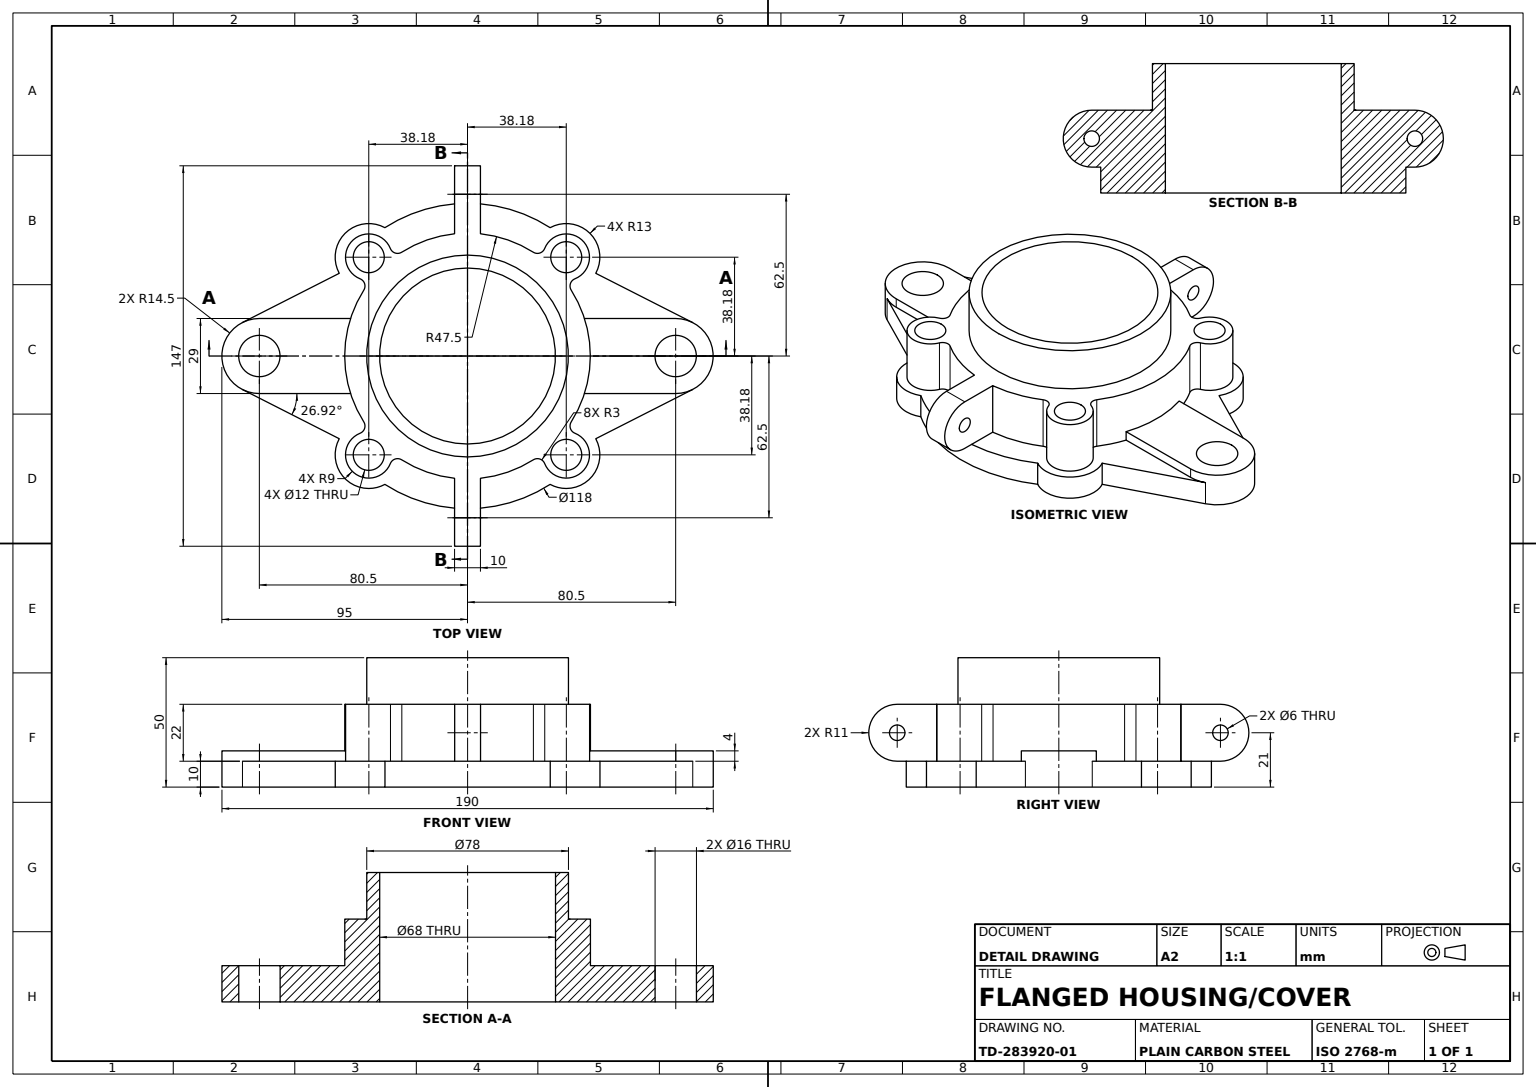
from build123d import *

# Parameters (mm, degrees)
BASE_FLANGE_SKETCH_R       = 59
BASE_FLANGE_118_DEPTH      = 10
FLANGE_LOBES_SKETCH_R      = 13
FLANGE_LOBES_DEPTH         = 10
HUB_AND_BOSSES_SKETCH_R    = 6
HUB_WITH_BOLT_BOSSES_DEPTH = 22
PIPE_COLLAR_SKETCH_R       = 39
PIPE_COLLAR_SKETCH_R_2     = 34
PIPE_COLLAR_78_DEPTH       = 18
SIDE_LUGS_DEPTH            = 22
LUG_GUSSET_A_SKETCH_R      = 3
LUG_GUSSET_A_DEPTH         = 10
LUG_HOLE_A_SKETCH_R        = 3
LUG_HOLE_A_DEPTH           = 10
LUG_GUSSET_B_SKETCH_R      = 3
LUG_GUSSET_B_DEPTH         = 10
LUG_HOLE_B_SKETCH_R        = 3
LUG_HOLE_B_DEPTH           = 10
MOUNTING_EARS_SKETCH_R     = 8
MOUNTING_EARS_DEPTH        = 10
EAR_RIB_A_SKETCH_R         = 8
EAR_RIB_A_DEPTH            = 4
EAR_RIB_B_SKETCH_R         = 8
EAR_RIB_B_DEPTH            = 4
SIDE_RELIEF_CUT_REACH      = 126.303
SIDE_RELIEF_CUT_SKETCH_R   = 6
PIPE_BORE_REACH            = 126.303
PIPE_BORE_SKETCH_R         = 34


with BuildPart() as part:
    # Base Flange Sketch → Base Flange Ø118 (new body)
    with BuildSketch(Plane(origin=(0, 0, 0), x_dir=(1, 0, 0), z_dir=(0, 1, 0))):
        with Locations(Location((0, 0, 0), (0, 0, 270))):
            Circle(BASE_FLANGE_SKETCH_R)
    extrude(amount=BASE_FLANGE_118_DEPTH)

    # Flange Lobes Sketch → Flange Lobes (add)
    with BuildSketch(Plane(origin=(0, 10, 0), x_dir=(1, 0, 0), z_dir=(0, 1, 0))):
        with Locations((-38.183766184, 38.183766184)):
            Circle(FLANGE_LOBES_SKETCH_R)
        with Locations((38.183766184, 38.183766184)):
            Circle(FLANGE_LOBES_SKETCH_R)
        with Locations((38.183766184, -38.183766184)):
            Circle(FLANGE_LOBES_SKETCH_R)
        with Locations((-38.183766184, -38.183766184)):
            Circle(FLANGE_LOBES_SKETCH_R)
    extrude(amount=-FLANGE_LOBES_DEPTH)

    # Hub and Bosses Sketch → Hub with Bolt Bosses (add)
    with BuildSketch(Plane(origin=(0, 10, 0), x_dir=(1, 0, 0), z_dir=(0, 1, 0))):
        with BuildLine():
            ThreePointArc((-40.114125183, 25.438297128), (-47.5, 0), (-40.114125183, -25.438297128))
            ThreePointArc((-40.114125183, -25.438297128), (-39.792711515, -27.966518872), (-41.531678205, -29.829636361))
            ThreePointArc((-41.531678205, -29.829636361), (-44.547727215, -44.547727215), (-29.829636361, -41.531678205))
            ThreePointArc((-29.829636361, -41.531678205), (-27.966518872, -39.792711515), (-25.438297128, -40.114125183))
            ThreePointArc((-25.438297128, -40.114125183), (0, -47.5), (25.438297128, -40.114125183))
            ThreePointArc((25.438297128, -40.114125183), (27.966518872, -39.792711515), (29.829636361, -41.531678205))
            ThreePointArc((29.829636361, -41.531678205), (44.547727215, -44.547727215), (41.531678205, -29.829636361))
            ThreePointArc((41.531678205, -29.829636361), (39.792711515, -27.966518872), (40.114125183, -25.438297128))
            ThreePointArc((40.114125183, -25.438297128), (47.5, 0), (40.114125183, 25.438297128))
            ThreePointArc((40.114125183, 25.438297128), (39.792711515, 27.966518872), (41.531678205, 29.829636361))
            ThreePointArc((41.531678205, 29.829636361), (44.547727215, 44.547727215), (29.829636361, 41.531678205))
            ThreePointArc((29.829636361, 41.531678205), (27.966518872, 39.792711515), (25.438297128, 40.114125183))
            ThreePointArc((25.438297128, 40.114125183), (0, 47.5), (-25.438297128, 40.114125183))
            ThreePointArc((-25.438297128, 40.114125183), (-27.966518872, 39.792711515), (-29.829636361, 41.531678205))
            ThreePointArc((-29.829636361, 41.531678205), (-44.547727215, 44.547727215), (-41.531678205, 29.829636361))
            ThreePointArc((-41.531678205, 29.829636361), (-39.792711515, 27.966518872), (-40.114125183, 25.438297128))
        make_face()
        with Locations(Location((-38.183766184, 38.183766184, 0), (0, 0, 270))):
            Circle(HUB_AND_BOSSES_SKETCH_R, mode=Mode.SUBTRACT)
        with Locations(Location((38.183766184, 38.183766184, 0), (0, 0, 270))):
            Circle(HUB_AND_BOSSES_SKETCH_R, mode=Mode.SUBTRACT)
        with Locations(Location((38.183766184, -38.183766184, 0), (0, 0, 270))):
            Circle(HUB_AND_BOSSES_SKETCH_R, mode=Mode.SUBTRACT)
        with Locations(Location((-38.183766184, -38.183766184, 0), (0, 0, 270))):
            Circle(HUB_AND_BOSSES_SKETCH_R, mode=Mode.SUBTRACT)
    extrude(amount=HUB_WITH_BOLT_BOSSES_DEPTH)

    # Pipe Collar Sketch → Pipe Collar Ø78 (add)
    with BuildSketch(Plane(origin=(0, 32, 0), x_dir=(1, 0, 0), z_dir=(0, 1, 0))):
        with Locations(Location((0, 0, 0), (0, 0, 270))):
            Circle(PIPE_COLLAR_SKETCH_R)
        with Locations(Location((0, 0, 0), (0, 0, 270))):
            Circle(PIPE_COLLAR_SKETCH_R_2, mode=Mode.SUBTRACT)
    extrude(amount=PIPE_COLLAR_78_DEPTH)

    # Side Lugs Sketch → Side Lugs (add)
    with BuildSketch(Plane(origin=(0, 10, 0), x_dir=(1, 0, 0), z_dir=(0, 1, 0))):
        with BuildLine():
            Line((-5, -47.236109069), (-5, -62.5))
            Line((-5, -62.5), (5, -62.5))
            Line((5, -62.5), (5, -47.236109069))
            ThreePointArc((5, -47.236109069), (0, -47.5), (-5, -47.236109069))
        make_face()
        with BuildLine():
            Line((-5, 47.236109069), (-5, 62.5))
            Line((-5, 62.5), (5, 62.5))
            Line((5, 62.5), (5, 47.236109069))
            ThreePointArc((5, 47.236109069), (0, 47.5), (-5, 47.236109069))
        make_face()
    extrude(amount=SIDE_LUGS_DEPTH)

    # Lug Gusset A Sketch → Lug Gusset A (add)
    with BuildSketch(Plane(origin=(5, 0, 0), x_dir=(0, 0, -1), z_dir=(1, 0, 0))):
        with BuildLine():
            Line((-62.5, 32), (-47.236109069, 32))
            Line((-47.236109069, 32), (-47.183766184, 10))
            Line((-47.183766184, 10), (-62.5, 10))
            ThreePointArc((-62.5, 10), (-73.5, 21), (-62.5, 32))
        make_face()
        with Locations((-62.5, 21)):
            Circle(LUG_GUSSET_A_SKETCH_R, mode=Mode.SUBTRACT)
    extrude(amount=-LUG_GUSSET_A_DEPTH)

    # Lug Hole A Sketch → Lug Hole A (cut)
    with BuildSketch(Plane(origin=(5, 0, 0), x_dir=(0, 0, -1), z_dir=(1, 0, 0))):
        with Locations((-62.5, 21)):
            Circle(LUG_HOLE_A_SKETCH_R)
    extrude(amount=-LUG_HOLE_A_DEPTH, mode=Mode.SUBTRACT)

    # Lug Gusset B Sketch → Lug Gusset B (add)
    with BuildSketch(Plane(origin=(5, 0, 0), x_dir=(0, 0, -1), z_dir=(1, 0, 0))):
        with BuildLine():
            Line((62.5, 32), (47.183766184, 32))
            Line((47.183766184, 32), (47.236109069, 10))
            Line((47.236109069, 10), (62.5, 10))
            ThreePointArc((62.5, 10), (73.5, 21), (62.5, 32))
        make_face()
        with Locations((62.5, 21)):
            Circle(LUG_GUSSET_B_SKETCH_R, mode=Mode.SUBTRACT)
    extrude(amount=-LUG_GUSSET_B_DEPTH)

    # Lug Hole B Sketch → Lug Hole B (cut)
    with BuildSketch(Plane(origin=(5, 0, 0), x_dir=(0, 0, -1), z_dir=(1, 0, 0))):
        with Locations((62.5, 21)):
            Circle(LUG_HOLE_B_SKETCH_R)
    extrude(amount=-LUG_HOLE_B_DEPTH, mode=Mode.SUBTRACT)

    # Mounting Ears Sketch → Mounting Ears (add)
    # profile 1 of 2: a face of its own
    with BuildSketch(Plane(origin=(0, 0, 0), x_dir=(1, 0, 0), z_dir=(0, 1, 0))):
        with BuildLine():
            Line((-87.065615201, 12.928367918), (-49.595662085, 31.957320012))
            ThreePointArc((-49.595662085, 31.957320012), (-59, 0), (-49.595662085, -31.957320012))
            Line((-49.595662085, -31.957320012), (-87.065615201, -12.928367918))
            ThreePointArc((-87.065615201, -12.928367918), (-95, 0), (-87.065615201, 12.928367918))
        make_face()
        with Locations(Location((-80.5, 0, 0), (0, 0, 270))):
            Circle(MOUNTING_EARS_SKETCH_R, mode=Mode.SUBTRACT)
    # profile 2 of 2: a face of its own
    with BuildSketch(Plane(origin=(0, 0, 0), x_dir=(1, 0, 0), z_dir=(0, 1, 0))):
        with BuildLine():
            Line((87.065615201, 12.928367918), (49.595662085, 31.957320012))
            ThreePointArc((49.595662085, 31.957320012), (59, 0), (49.595662085, -31.957320012))
            Line((49.595662085, -31.957320012), (87.065615201, -12.928367918))
            ThreePointArc((87.065615201, -12.928367918), (95, 0), (87.065615201, 12.928367918))
        make_face()
        with Locations(Location((80.5, 0, 0), (0, 0, 270))):
            Circle(MOUNTING_EARS_SKETCH_R, mode=Mode.SUBTRACT)
    extrude(amount=MOUNTING_EARS_DEPTH)

    # Ear Rib A Sketch → Ear Rib A (add)
    with BuildSketch(Plane(origin=(0, 10, 0), x_dir=(1, 0, 0), z_dir=(0, 1, 0))):
        with BuildLine():
            Line((-80.5, 14.5), (-45.232731512, 14.5))
            ThreePointArc((-45.232731512, 14.5), (-47.5, 0), (-45.232731512, -14.5))
            Line((-45.232731512, -14.5), (-80.5, -14.5))
            ThreePointArc((-80.5, -14.5), (-95, 0), (-80.5, 14.5))
        make_face()
        with Locations(Location((-80.5, 0, 0), (0, 0, 270))):
            Circle(EAR_RIB_A_SKETCH_R, mode=Mode.SUBTRACT)
    extrude(amount=EAR_RIB_A_DEPTH)

    # Ear Rib B Sketch → Ear Rib B (add)
    with BuildSketch(Plane(origin=(0, 10, 0), x_dir=(1, 0, 0), z_dir=(0, 1, 0))):
        with BuildLine():
            Line((80.5, 14.5), (45.232731512, 14.5))
            ThreePointArc((45.232731512, 14.5), (47.5, 0), (45.232731512, -14.5))
            Line((45.232731512, -14.5), (80.5, -14.5))
            ThreePointArc((80.5, -14.5), (95, 0), (80.5, 14.5))
        make_face()
        with Locations(Location((80.5, 0, 0), (0, 0, 270))):
            Circle(EAR_RIB_B_SKETCH_R, mode=Mode.SUBTRACT)
    extrude(amount=EAR_RIB_B_DEPTH)

    # Side Relief Cut Sketch → Side Relief Cut (cut, up to next)
    with BuildSketch(Plane(origin=(0, 32, 0), x_dir=(1, 0, 0), z_dir=(0, 1, 0)), mode=Mode.PRIVATE) as side_relief_cut_sk1:
        with Locations(Location((-38.183766184, 38.183766184, 0), (0, 0, 270))):
            Circle(SIDE_RELIEF_CUT_SKETCH_R)
    side_relief_cut_tool1 = extrude(side_relief_cut_sk1.sketch, amount=-SIDE_RELIEF_CUT_REACH, mode=Mode.PRIVATE) & part.part
    # Side Relief Cut Sketch → Side Relief Cut (cut, up to next)
    with BuildSketch(Plane(origin=(0, 32, 0), x_dir=(1, 0, 0), z_dir=(0, 1, 0)), mode=Mode.PRIVATE) as side_relief_cut_sk2:
        with Locations(Location((38.183766184, 38.183766184, 0), (0, 0, 270))):
            Circle(SIDE_RELIEF_CUT_SKETCH_R)
    side_relief_cut_tool2 = extrude(side_relief_cut_sk2.sketch, amount=-SIDE_RELIEF_CUT_REACH, mode=Mode.PRIVATE) & part.part
    # Side Relief Cut Sketch → Side Relief Cut (cut, up to next)
    with BuildSketch(Plane(origin=(0, 32, 0), x_dir=(1, 0, 0), z_dir=(0, 1, 0)), mode=Mode.PRIVATE) as side_relief_cut_sk3:
        with Locations(Location((38.183766184, -38.183766184, 0), (0, 0, 270))):
            Circle(SIDE_RELIEF_CUT_SKETCH_R)
    side_relief_cut_tool3 = extrude(side_relief_cut_sk3.sketch, amount=-SIDE_RELIEF_CUT_REACH, mode=Mode.PRIVATE) & part.part
    # Side Relief Cut Sketch → Side Relief Cut (cut, up to next)
    with BuildSketch(Plane(origin=(0, 32, 0), x_dir=(1, 0, 0), z_dir=(0, 1, 0)), mode=Mode.PRIVATE) as side_relief_cut_sk4:
        with Locations(Location((-38.183766184, -38.183766184, 0), (0, 0, 270))):
            Circle(SIDE_RELIEF_CUT_SKETCH_R)
    side_relief_cut_tool4 = extrude(side_relief_cut_sk4.sketch, amount=-SIDE_RELIEF_CUT_REACH, mode=Mode.PRIVATE) & part.part
    add(side_relief_cut_tool1.solids().sort_by_distance((-38.183766, 32, -38.183766))[0], mode=Mode.SUBTRACT)
    add(side_relief_cut_tool2.solids().sort_by_distance((38.183766, 32, -38.183766))[0], mode=Mode.SUBTRACT)
    add(side_relief_cut_tool3.solids().sort_by_distance((38.183766, 32, 38.183766))[0], mode=Mode.SUBTRACT)
    add(side_relief_cut_tool4.solids().sort_by_distance((-38.183766, 32, 38.183766))[0], mode=Mode.SUBTRACT)

    # Pipe Bore Sketch → Pipe Bore (cut, up to next)
    with BuildSketch(Plane(origin=(0, 32, 0), x_dir=(1, 0, 0), z_dir=(0, 1, 0)), mode=Mode.PRIVATE) as pipe_bore_sk1:
        with Locations(Location((0, 0, 0), (0, 0, 270))):
            Circle(PIPE_BORE_SKETCH_R)
    pipe_bore_tool1 = extrude(pipe_bore_sk1.sketch, amount=-PIPE_BORE_REACH, mode=Mode.PRIVATE) & part.part
    add(pipe_bore_tool1.solids().sort_by_distance((0, 32, 0))[0], mode=Mode.SUBTRACT)


solid = part.part
